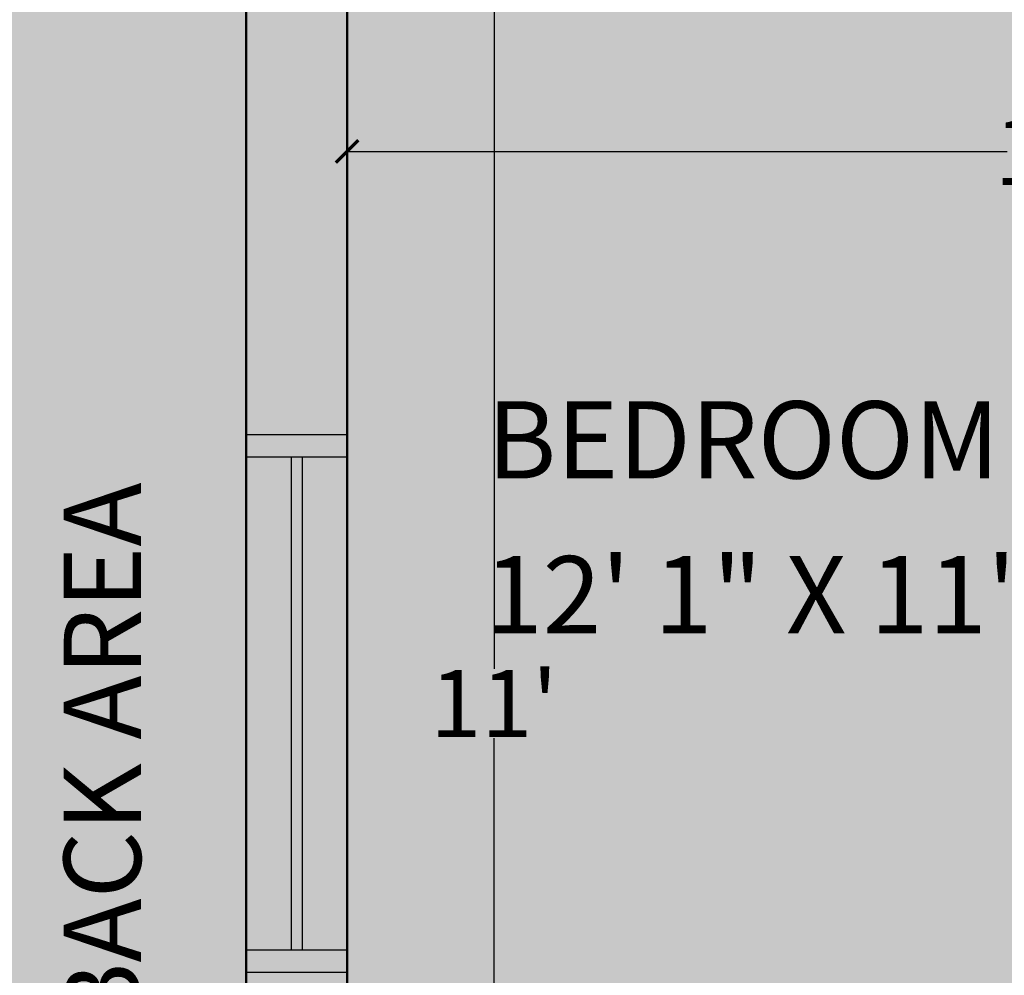
# Model space of a CAD drawing. Units: inches. Extents: x 528 to 2620, y -1066 to 798.
# Tile 7 of 41: x 600 to 688, y 620 to 705. Entities that reach past the tile are written whole.
import ezdxf

# ---------------------------------------------------------------- set-up
doc = ezdxf.new("R2010")
doc.units = ezdxf.units.IN
doc.header["$MEASUREMENT"] = 0
for name, color, linetype, lineweight in [('A-ANNO-DIMS', 2, 'Continuous', 18), ('A-AREA-IDEN', 7, 'Continuous', 18), ('A-GLAZ', 3, 'Continuous', 25), ('A-WALL', 7, 'Continuous', 50), ('A-WALL-PATT', 8, 'Continuous', 13)]:
    doc.layers.add(name, color=color, linetype=linetype, lineweight=lineweight)
doc.styles.get("Standard").update_dxf_attribs({"font": 'arial.ttf'})
doc.dimstyles.get("Standard").update_dxf_attribs({"dimtxt": 6, "dimasz": 2, "dimexe": 0.18, "dimexo": 0.0625, "dimgap": 0.09, "dimtad": 0, "dimtih": 1, "dimtoh": 1, "dimdec": 1, "dimzin": 0, "dimdsep": 46, "dimlunit": 3, "dimtxsty": 'Standard', "dimblk": 'ARCHTICK', "dimcen": 0.09, "dimadec": 0, "dimazin": 0, "dimtfac": 1, "dimtdec": 1, "dimtofl": 0, "dimtmove": 0, "dimatfit": 3, "dimfxl": 1, "dimtolj": 1, "dimtzin": 0, "dimarcsym": 0})

# ---------------------------------------------------------------- blocks, each defined once
blk = doc.blocks.new('_ArchTick')
at = {"color": 0, "linetype": 'ByBlock', "const_width": 0.15}
blk.add_lwpolyline([(-0.5, -0.5), (0.5, 0.5)], dxfattribs=at)
blk = doc.blocks.new('*D25')
at = {"layer": 'A-ANNO-DIMS', "color": 0, "lineweight": -2, "transparency": 16777216}
for p, q in [((629.059, 693.763), (629.059, 693.001)), ((774.059, 693.763), (774.059, 693.001)), ((629.059, 693.181), (687.951, 693.181)), ((774.059, 693.181), (715.168, 693.181))]:
    blk.add_line(p, q, dxfattribs=at)
at = {"layer": 'Defpoints', "color": 0, "transparency": 16777216}
for p in [(629.059, 693.826), (774.059, 693.826), (774.059, 693.181)]:
    blk.add_point(p, dxfattribs=at)
at = {"layer": 'A-ANNO-DIMS', "color": 0, "lineweight": -2, "transparency": 16777216, "xscale": 2, "yscale": 2, "zscale": 2, "rotation": 180}
blk.add_blockref('_ArchTick', (629.059, 693.181), dxfattribs=at)
at = {"layer": 'A-ANNO-DIMS', "color": 0, "lineweight": -2, "transparency": 16777216, "xscale": 2, "yscale": 2, "zscale": 2}
blk.add_blockref('_ArchTick', (774.059, 693.181), dxfattribs=at)
at = {"layer": 'A-ANNO-DIMS', "color": 0, "transparency": 16777216, "insert": (701.559, 693.181), "char_height": 6, "attachment_point": 5}
blk.add_mtext('\\A1;12\'-1.0"', dxfattribs=at)
blk = doc.blocks.new('*D26')
at = {"layer": 'A-ANNO-DIMS', "color": 0, "lineweight": -2, "transparency": 16777216}
for p, q in [((642.51, 709.922), (641.988, 709.922)), ((642.168, 709.922), (642.168, 647.025)), ((642.168, 577.922), (642.168, 640.82)), ((642.51, 577.922), (641.988, 577.922))]:
    blk.add_line(p, q, dxfattribs=at)
at = {"layer": 'Defpoints', "color": 0, "transparency": 16777216}
for p in [(642.572, 709.922), (642.168, 577.922), (642.572, 577.922)]:
    blk.add_point(p, dxfattribs=at)
at = {"layer": 'A-ANNO-DIMS', "color": 0, "lineweight": -2, "transparency": 16777216, "xscale": 2, "yscale": 2, "zscale": 2}
for p, rotation in [((642.168, 709.922), 90), ((642.168, 577.922), 270)]:
    blk.add_blockref('_ArchTick', p, dxfattribs=dict(at, rotation=rotation))
at = {"layer": 'A-ANNO-DIMS', "color": 0, "transparency": 16777216, "insert": (642.168, 643.922), "char_height": 6, "attachment_point": 5}
blk.add_mtext("\\A1;11'", dxfattribs=at)
blk = doc.blocks.new('WIN-1200')
for p, q in [((677.559, 718.922), (725.559, 718.922)), ((677.559, 709.922), (677.559, 718.922)), ((679.559, 709.922), (679.559, 718.922)), ((723.559, 718.922), (723.559, 709.922)), ((725.559, 718.922), (725.559, 709.922)), ((679.559, 714.922), (723.559, 714.922)), ((679.559, 713.922), (723.559, 713.922)), ((725.559, 709.922), (677.559, 709.922))]:
    blk.add_line(p, q)

msp = doc.modelspace()

# ---------------------------------------------------------------- hatches: boundary and pattern name
at = {"layer": 'A-WALL-PATT', "transparency": 33554475}
h = msp.add_hatch(color=256, dxfattribs=at)
h.dxf.hatch_style = 1
h.paths.add_polyline_path([(620.059, 718.922), (908.059, 718.922), (908.059, 268.922), (770.059, 268.922), (770.059, 220.922), (932.059, 220.922), (932.059, 741.922), (596.059, 741.922), (596.059, 391.422), (620.059, 391.422)])
at = {"layer": 'A-WALL-PATT', "transparency": 33554687}
h = msp.add_hatch(color=256, dxfattribs=at)
h.dxf.hatch_style = 1
h.paths.add_polyline_path([(861.059, 273.922), (817.059, 273.922), (817.059, 272.922), (861.059, 272.922)])
h.paths.add_polyline_path([(817.059, 277.922), (815.059, 277.922), (815.059, 268.922), (817.059, 268.922)])
h.paths.add_polyline_path([(908.059, 397.922), (899.059, 397.922), (899.059, 395.922), (908.059, 395.922)])
h.paths.add_polyline_path([(908.059, 443.922), (899.059, 443.922), (899.059, 441.922), (908.059, 441.922)])
h.paths.add_polyline_path([(904.059, 441.922), (903.059, 441.922), (903.059, 397.922), (904.059, 397.922)])
h.paths.add_polyline_path([(625.059, 561.422), (624.059, 561.422), (624.059, 537.422), (625.059, 537.422)])
h.paths.add_polyline_path([(648.747, 334.444), (720.045, 334.444), (720.045, 344.998), (648.747, 344.998)], flags=9)
h.paths.add_polyline_path([(819.733, 323.153), (880.328, 323.153), (880.328, 333.708), (819.733, 333.708)], flags=9)
h.paths.add_polyline_path([(779.898, 680.607), (821.764, 680.607), (821.764, 691.169), (779.898, 691.169)], flags=9)
h.paths.add_polyline_path([(779.876, 692.362), (817.138, 692.362), (817.138, 703.058), (779.876, 703.058)], flags=9)
h.paths.add_polyline_path([(799.994, 453.884), (860.589, 453.884), (860.589, 464.439), (799.994, 464.439)], flags=9)
h.paths.add_polyline_path([(650.866, 539.397), (708.781, 539.397), (708.781, 549.952), (650.866, 549.952)], flags=9)
h.paths.add_polyline_path([(788.504, 612.01), (849.099, 612.01), (849.099, 622.565), (788.504, 622.565)], flags=9)
h.paths.add_polyline_path([(639.539, 648.31), (700.134, 648.31), (700.134, 658.865), (639.539, 658.865)], flags=9)
h.paths.add_polyline_path([(648.913, 346.09), (747.706, 346.09), (747.706, 356.778), (648.913, 356.778)], flags=9)
h.paths.add_polyline_path([(676.857, 450.66), (746.735, 450.66), (746.735, 461.355), (676.857, 461.355)], flags=9)
h.paths.add_polyline_path([(819.711, 334.947), (865.526, 334.947), (865.526, 345.636), (819.711, 345.636)], flags=9)
h.paths.add_polyline_path([(806.298, 467.745), (874.047, 467.745), (874.047, 478.441), (806.298, 478.441)], flags=9)
h.paths.add_polyline_path([(653.235, 552.284), (690.497, 552.284), (690.497, 562.979), (653.235, 562.979)], flags=9)
h.paths.add_polyline_path([(789.903, 623.407), (843.208, 623.407), (843.208, 634.103), (789.903, 634.103)], flags=9)
h.paths.add_polyline_path([(639.773, 662.103), (693.077, 662.103), (693.077, 672.798), (639.773, 672.798)], flags=9)
h.paths.add_polyline_path([(801.587, 242.914), (846.334, 242.914), (846.334, 253.603), (801.587, 253.603)], flags=9)
h.paths.add_polyline_path([(925.362, 593.982), (925.362, 674.057), (914.673, 674.057), (914.673, 593.982)], flags=9)
h.paths.add_polyline_path([(612.559, 593.982), (612.559, 674.057), (601.871, 674.057), (601.871, 593.982)], flags=9)
h.paths.add_polyline_path([(723.31, 726.564), (803.385, 726.564), (803.385, 737.252), (723.31, 737.252)], flags=9)
at = {"layer": 'A-WALL-PATT', "transparency": 33554521}
h = msp.add_hatch(color=256, dxfattribs=at)
h.dxf.hatch_style = 1
h.paths.add_polyline_path([(629.059, 709.922), (677.559, 709.922), (677.559, 718.922), (620.059, 718.922), (620.059, 667.922), (629.059, 667.922)])
h.paths.add_polyline_path([(790.559, 718.922), (725.559, 718.922), (725.559, 709.922), (774.059, 709.922), (774.059, 577.922), (768.481, 577.922), (768.559, 573.422), (774.059, 573.422), (774.059, 567.422), (778.559, 567.422), (778.559, 669.422), (831.059, 669.422), (831.059, 675.922), (826.559, 675.922), (826.559, 673.922), (778.559, 673.922), (778.559, 709.922), (790.559, 709.922)])
h.paths.add_polyline_path([(908.059, 718.922), (879.059, 718.922), (879.059, 709.922), (899.059, 709.922), (899.059, 641.672), (908.059, 641.672)])
h.paths.add_polyline_path([(629.059, 619.922), (620.059, 619.922), (620.059, 561.422), (629.059, 561.422), (629.059, 573.422), (724.059, 573.422), (724.059, 569.422), (728.559, 569.422), (728.559, 577.922), (629.059, 577.922)])
h.paths.add_polyline_path([(779.059, 391.422), (779.059, 400.422), (770.059, 400.422), (764.059, 400.422), (764.059, 397.422), (764.059, 391.422), (770.059, 391.422), (770.059, 268.922), (815.059, 268.922), (815.059, 277.922), (779.059, 277.922), (779.059, 359.767)])
h.paths.add_polyline_path([(908.059, 395.922), (899.059, 395.922), (851.059, 395.922), (851.059, 391.422), (899.059, 391.422), (899.059, 277.922), (863.059, 277.922), (863.059, 268.922), (908.059, 268.922)])
h.paths.add_polyline_path([(908.059, 593.672), (899.059, 593.672), (899.059, 525.422), (778.559, 525.422), (778.559, 527.172), (774.059, 527.172), (774.059, 520.922), (899.059, 520.922), (899.059, 443.922), (908.059, 443.922)])
h.paths.add_polyline_path([(629.059, 520.922), (728.559, 520.922), (728.559, 545.422), (724.059, 545.422), (724.059, 525.422), (629.059, 525.422), (629.059, 537.422), (620.059, 537.422), (620.059, 484.672), (629.059, 484.672)])
h.paths.add_polyline_path([(629.059, 436.672), (620.059, 436.672), (620.059, 391.422), (648.559, 391.422), (648.559, 400.422), (629.059, 400.422)])
h.paths.add_polyline_path([(716.059, 397.422), (716.059, 400.422), (696.559, 400.422), (696.559, 391.422), (716.059, 391.422)])
at = {"layer": 'A-WALL-PATT', "transparency": 33554681}
h = msp.add_hatch(color=256, dxfattribs=at)
h.dxf.hatch_style = 1
h.paths.add_polyline_path([(629.059, 665.922), (625.059, 665.922), (625.059, 621.922), (629.059, 621.922)])
h.paths.add_polyline_path([(624.059, 665.922), (620.059, 665.922), (620.059, 621.922), (624.059, 621.922)])
h.paths.add_polyline_path([(723.559, 713.922), (679.559, 713.922), (679.559, 709.922), (723.559, 709.922)])
h.paths.add_polyline_path([(723.559, 718.922), (679.559, 718.922), (679.559, 714.922), (723.559, 714.922)])
h.paths.add_polyline_path([(814.559, 713.922), (790.559, 713.922), (790.559, 709.922), (814.559, 709.922)])
h.paths.add_polyline_path([(814.559, 718.922), (790.559, 718.922), (790.559, 714.922), (814.559, 714.922)])
h.paths.add_polyline_path([(877.059, 713.922), (833.059, 713.922), (833.059, 709.922), (877.059, 709.922)])
h.paths.add_polyline_path([(877.059, 718.922), (833.059, 718.922), (833.059, 714.922), (877.059, 714.922)])
h.paths.add_polyline_path([(908.059, 639.672), (904.059, 639.672), (904.059, 595.672), (908.059, 595.672)])
h.paths.add_polyline_path([(903.059, 639.672), (899.059, 639.672), (899.059, 595.672), (903.059, 595.672)])
h.paths.add_polyline_path([(908.059, 441.922), (904.059, 441.922), (904.059, 397.922), (908.059, 397.922)])
h.paths.add_polyline_path([(903.059, 441.922), (899.059, 441.922), (899.059, 397.922), (903.059, 397.922)])
h.paths.add_polyline_path([(861.059, 272.922), (817.059, 272.922), (817.059, 268.922), (861.059, 268.922)])
h.paths.add_polyline_path([(861.059, 277.922), (817.059, 277.922), (817.059, 273.922), (861.059, 273.922)])
h.paths.add_polyline_path([(694.559, 395.422), (650.559, 395.422), (650.559, 391.422), (694.559, 391.422)])
h.paths.add_polyline_path([(694.559, 400.422), (650.559, 400.422), (650.559, 396.422), (694.559, 396.422)])
h.paths.add_polyline_path([(629.059, 482.672), (625.059, 482.672), (625.059, 438.672), (629.059, 438.672)])
h.paths.add_polyline_path([(624.059, 482.672), (620.059, 482.672), (620.059, 438.672), (624.059, 438.672)])
h.paths.add_polyline_path([(629.059, 561.422), (625.059, 561.422), (625.059, 537.422), (629.059, 537.422)])
h.paths.add_polyline_path([(624.059, 561.422), (620.059, 561.422), (620.059, 537.422), (624.059, 537.422)])
h = msp.add_hatch(color=256, dxfattribs=at)
h.dxf.hatch_style = 1
h.paths.add_polyline_path([(625.059, 665.922), (624.059, 665.922), (624.059, 621.922), (625.059, 621.922)])
h.paths.add_polyline_path([(629.059, 667.922), (620.059, 667.922), (620.059, 665.922), (629.059, 665.922)])
h.paths.add_polyline_path([(629.059, 621.922), (620.059, 621.922), (620.059, 619.922), (629.059, 619.922)])
h.paths.add_polyline_path([(723.559, 714.922), (679.559, 714.922), (679.559, 713.922), (723.559, 713.922)])
h.paths.add_polyline_path([(725.559, 718.922), (723.559, 718.922), (723.559, 709.922), (725.559, 709.922)])
h.paths.add_polyline_path([(679.559, 718.922), (677.559, 718.922), (677.559, 709.922), (679.559, 709.922)])
h.paths.add_polyline_path([(814.559, 714.922), (790.559, 714.922), (790.559, 713.922), (814.559, 713.922)])
h.paths.add_polyline_path([(877.059, 714.922), (833.059, 714.922), (833.059, 713.922), (877.059, 713.922)])
h.paths.add_polyline_path([(879.059, 718.922), (877.059, 718.922), (877.059, 709.922), (879.059, 709.922)])
h.paths.add_polyline_path([(833.059, 718.922), (831.059, 718.922), (831.059, 709.922), (833.059, 709.922)])
h.paths.add_polyline_path([(650.559, 400.422), (648.559, 400.422), (648.559, 391.422), (650.559, 391.422)])
h.paths.add_polyline_path([(694.559, 396.422), (650.559, 396.422), (650.559, 395.422), (694.559, 395.422)])
h.paths.add_polyline_path([(696.559, 400.422), (694.559, 400.422), (694.559, 391.422), (696.559, 391.422)])
h.paths.add_polyline_path([(629.059, 438.672), (620.059, 438.672), (620.059, 436.672), (629.059, 436.672)])
h.paths.add_polyline_path([(629.059, 484.672), (620.059, 484.672), (620.059, 482.672), (629.059, 482.672)])
h.paths.add_polyline_path([(625.059, 482.672), (624.059, 482.672), (624.059, 438.672), (625.059, 438.672)])
at = {"layer": 'A-WALL-PATT', "transparency": 33554590}
h = msp.add_hatch(color=256, dxfattribs=at)
h.dxf.hatch_style = 1
h.paths.add_polyline_path([(774.059, 709.922), (629.059, 709.922), (629.059, 577.922), (728.559, 577.922), (728.559, 579.422), (728.559, 619.422), (730.309, 619.422), (730.309, 619.384, -0.401453), (768.559, 579.422), (768.559, 577.922), (774.059, 577.922)])
h.paths.add_polyline_path([(723.896, 686.058), (723.968, 686.064), (723.828, 686.128)], flags=0)
h.paths.add_polyline_path([(722.785, 642.699), (722.893, 642.756), (722.893, 684.992), (722.647, 685.244), (722.647, 685.82), (723.079, 686.262), (723.533, 686.262), (723.968, 686.064), (724.739, 686.128), (770.696, 686.128), (770.78, 686.14), (771.126, 686.266), (771.694, 686.094), (771.94, 685.478), (771.67, 684.904), (771.582, 684.871), (771.582, 642.782), (771.878, 642.514), (771.878, 641.921), (771.511, 641.462), (770.855, 641.462), (770.401, 641.833), (770.401, 641.551), (724.739, 641.551), (723.991, 641.705), (723.443, 641.414), (722.879, 641.585), (722.597, 642.142)], flags=16)
h.paths.add_polyline_path([(723.994, 641.704), (723.994, 641.707), (723.991, 641.705)], flags=0)
h.paths.add_polyline_path([(722.893, 642.732), (722.893, 684.992), (722.647, 685.244), (722.647, 685.82), (723.079, 686.262), (723.287, 686.262), (722.991, 686.172), (722.794, 685.971), (722.647, 685.68), (722.647, 685.434), (722.745, 685.143), (722.942, 684.942), (723.238, 684.807), (723.484, 684.807), (723.779, 684.897), (723.976, 685.098), (724.174, 685.488), (724.124, 685.635), (724.124, 685.249), (723.631, 684.746), (723.631, 642.961), (724.124, 642.514), (724.124, 641.887), (723.656, 641.462), (723.079, 641.462), (722.647, 641.904), (722.647, 642.48)], flags=0)
h.paths.add_polyline_path([(722.647, 642.29), (722.647, 642.044), (722.794, 641.753), (723.079, 641.462), (723.287, 641.462), (722.879, 641.585), (722.597, 642.142)], flags=0)
h.paths.add_polyline_path([(770.745, 686.128), (770.58, 686.128), (770.551, 686.057)], flags=0)
h.paths.add_polyline_path([(743.299, 645.288), (753.227, 659.398), (748.69, 663.75), (753.234, 668.538), (743.299, 682.458), (743.791, 682.592), (744.136, 682.681), (744.53, 682.928), (744.628, 683.084), (745.017, 683.327), (744.53, 684.069), (744.776, 684.158), (744.874, 684.315), (745.514, 684.404), (746.081, 684.651), (746.474, 684.651), (746.819, 684.807), (747.459, 685.031), (747.705, 685.143), (748.198, 685.277), (748.394, 685.523), (748.862, 685.523), (749.994, 686.128), (753.488, 676.03), (757.379, 680.153), (757.791, 679.758), (758.044, 680.645), (758.29, 681.227), (758.29, 682.055), (758.019, 682.592), (757.871, 683.174), (757.822, 683.778), (758.388, 684.069), (758.979, 684.203), (759.619, 684.158), (760.21, 683.957), (760.751, 683.666), (761.859, 683.666), (762.401, 683.957), (762.991, 684.114), (763.631, 684.114), (764.198, 683.957), (764.739, 683.666), (766.118, 683.666), (766.659, 683.957), (767.25, 684.158), (767.865, 684.203), (768.456, 684.069), (769.047, 683.778), (768.998, 683.174), (768.85, 682.592), (768.554, 682.055), (768.554, 681.227), (768.801, 680.645), (769.092, 679.75), (768.948, 678.832), (768.801, 678.228), (768.554, 677.646), (768.554, 676.818), (768.801, 676.237), (769.092, 675.341), (768.948, 674.424), (768.801, 673.82), (768.554, 673.283), (768.554, 672.41), (768.801, 671.873), (768.998, 671.291), (769.047, 670.642), (768.948, 670.016), (768.801, 669.411), (768.554, 668.874), (768.554, 668.002), (768.974, 667.239), (769.047, 666.279), (769.047, 665.563), (768.456, 665.316), (767.865, 665.16), (767.25, 665.16), (766.659, 665.361), (766.118, 665.697), (764.739, 665.697), (763.945, 665.204), (762.991, 665.204), (762.401, 665.361), (761.859, 665.697), (761.005, 665.697), (762.696, 664.086), (760.741, 662.027), (761.859, 662.027), (762.401, 662.318), (763.342, 662.548), (764.247, 662.318), (764.788, 662.027), (766.118, 662.027), (766.659, 662.318), (767.25, 662.519), (767.865, 662.564), (768.505, 662.43), (769.047, 662.116), (769.047, 661.4), (769.047, 660.796), (768.85, 660.214), (768.554, 659.677), (768.554, 658.849), (768.85, 658.267), (768.998, 657.663), (769.069, 656.749), (768.85, 655.851), (768.554, 655.269), (768.554, 654.441), (768.85, 653.859), (769.069, 652.961), (768.998, 652.046), (768.85, 651.442), (768.554, 650.905), (768.554, 650.032), (768.85, 649.495), (768.998, 648.914), (769.047, 648.265), (768.998, 647.638), (768.85, 647.034), (768.554, 646.497), (768.554, 645.624), (768.85, 645.087), (769.047, 644.55), (769.047, 643.901), (768.505, 643.655), (767.865, 643.521), (767.25, 643.521), (766.659, 643.722), (766.118, 644.058), (764.788, 644.058), (764.247, 643.722), (763.342, 643.492), (762.401, 643.722), (761.859, 644.058), (760.801, 644.058), (760.259, 643.722), (759.668, 643.521), (759.028, 643.521), (758.388, 643.655), (757.871, 643.901), (757.871, 644.55), (758.044, 645.087), (758.339, 645.624), (758.339, 646.497), (758.044, 647.034), (757.921, 647.638), (757.866, 648.059), (757.379, 647.593), (753.422, 651.773), (749.994, 641.618), (749.502, 641.708), (749.354, 641.954), (748.542, 642.446), (747.311, 642.939), (746.652, 642.939), (746.327, 643.185), (745.514, 643.565), (744.53, 643.655), (745.011, 644.4), (744.628, 644.639), (744.136, 644.886), (743.791, 645.132)], flags=0)
h.paths.add_polyline_path([(755.656, 654.933), (756.542, 654.687), (757.527, 654.329), (756.641, 654.575)], flags=0)
h.paths.add_polyline_path([(758.339, 649.204), (758.339, 648.712), (758.585, 644.304), (758.585, 648.802)], flags=0)
h.paths.add_polyline_path([(758.339, 649.294), (758.093, 649.697), (758.359, 649.165)], flags=0)
h.paths.add_polyline_path([(755.656, 672.79), (756.493, 673.037), (757.358, 673.351), (757.353, 673.358), (756.641, 673.149)], flags=0)
h.paths.add_polyline_path([(760.264, 639.641), (771.408, 639.641), (771.408, 624.039), (760.264, 624.039)], flags=16)
h.paths.add_polyline_path([(761.378, 638.526), (770.294, 638.526), (770.294, 625.153), (761.378, 625.153)], flags=0)
edge = h.paths.add_edge_path(flags=0)
edge.add_ellipse((765.836, 631.84), major_axis=(-2.245, 2.245), ratio=1, start_angle=-45, end_angle=45, ccw=False)
edge.add_ellipse((765.836, 631.84), major_axis=(-2.245, 2.245), ratio=1, start_angle=-135, end_angle=-45, ccw=False)
edge.add_ellipse((765.836, 631.84), major_axis=(-2.245, 2.245), ratio=1, start_angle=135, end_angle=-135, ccw=False)
edge.add_ellipse((765.836, 631.84), major_axis=(-2.245, 2.245), ratio=1, start_angle=45, end_angle=135, ccw=False)
h.paths.add_polyline_path([(758.585, 683.42), (758.585, 678.922), (758.373, 678.575), (758.339, 678.43), (758.093, 678.049), (758.339, 678.519), (758.339, 679.011)], flags=0)
h.paths.add_polyline_path([(760.264, 688.038), (760.264, 703.64), (771.408, 703.64), (771.408, 688.038)], flags=16)
h.paths.add_polyline_path([(770.401, 685.389), (770.401, 685.846), (770.855, 686.217), (771.511, 686.217), (771.878, 685.758), (771.878, 685.165), (771.582, 684.897), (771.582, 642.782), (771.878, 642.514), (771.878, 641.921), (771.511, 641.462), (770.855, 641.462), (770.401, 641.833), (770.401, 642.29)], flags=0)
h.paths.add_polyline_path([(770.532, 642.678), (771.052, 643.009), (771.67, 642.775), (771.94, 642.201), (771.694, 641.585), (771.126, 641.413), (770.551, 641.622), (770.347, 642.132)], flags=16)
h.paths.add_polyline_path([(761.378, 689.152), (761.378, 702.526), (770.294, 702.526), (770.294, 689.152)], flags=0)
edge = h.paths.add_edge_path(flags=0)
edge.add_ellipse((765.836, 695.839), major_axis=(2.245, 2.245), ratio=1, start_angle=405, end_angle=495, ccw=False)
edge.add_ellipse((765.836, 695.839), major_axis=(2.245, 2.245), ratio=1, start_angle=675, end_angle=765, ccw=False)
edge.add_ellipse((765.836, 695.839), major_axis=(2.245, 2.245), ratio=1, start_angle=585, end_angle=675, ccw=False)
edge.add_ellipse((765.836, 695.839), major_axis=(2.245, 2.245), ratio=1, start_angle=495, end_angle=585, ccw=False)
h.paths.add_polyline_path([(770.696, 684.897), (770.942, 684.74), (771.41, 684.74), (771.73, 685.031), (771.878, 685.344), (771.878, 685.635), (771.694, 686.094), (771.582, 686.128), (771.878, 685.758), (771.878, 685.165), (771.41, 684.74), (770.849, 684.74)], flags=0)
h.paths.add_polyline_path([(899.059, 709.922), (831.059, 709.922), (831.059, 699.922), (829.809, 699.922), (829.809, 675.922), (831.059, 675.922), (831.059, 669.422), (778.559, 669.422), (778.559, 567.172), (780.059, 567.172), (820.059, 567.172), (820.059, 565.422), (820.021, 565.422, -0.401453), (780.059, 527.172), (778.559, 527.172), (778.559, 525.422), (899.059, 525.422)])
h.paths.add_polyline_path([(849.197, 636.014), (849.269, 636.02), (849.129, 636.084)], flags=0)
h.paths.add_polyline_path([(848.193, 634.948), (847.947, 635.2), (847.947, 635.776), (848.379, 636.218), (848.833, 636.218), (849.269, 636.02), (850.039, 636.084), (895.996, 636.084), (896.081, 636.096), (896.426, 636.222), (896.995, 636.05), (897.241, 635.434), (896.97, 634.86), (896.883, 634.827), (896.883, 592.738), (897.178, 592.47), (897.178, 591.877), (896.811, 591.418), (896.155, 591.418), (895.701, 591.789), (895.701, 591.507), (850.039, 591.507), (849.292, 591.661), (848.744, 591.37), (848.18, 591.541), (847.897, 592.098), (848.086, 592.655), (848.193, 592.712)], flags=16)
h.paths.add_polyline_path([(849.294, 591.66), (849.295, 591.663), (849.292, 591.661)], flags=16)
h.paths.add_polyline_path([(848.193, 634.948), (847.947, 635.2), (847.947, 635.776), (848.379, 636.218), (848.587, 636.218), (848.292, 636.128), (848.095, 635.927), (847.947, 635.636), (847.947, 635.39), (848.046, 635.099), (848.243, 634.897), (848.538, 634.763), (848.784, 634.763), (849.079, 634.853), (849.276, 635.054), (849.474, 635.444), (849.424, 635.591), (849.424, 635.205), (848.932, 634.702), (848.932, 592.917), (849.424, 592.47), (849.424, 591.843), (848.956, 591.418), (848.379, 591.418), (847.947, 591.86), (847.947, 592.436), (848.193, 592.688)], flags=0)
h.paths.add_polyline_path([(847.947, 592.246), (847.947, 592), (848.095, 591.709), (848.379, 591.418), (848.587, 591.418), (848.18, 591.541), (847.897, 592.098)], flags=16)
h.paths.add_polyline_path([(896.046, 636.084), (895.88, 636.084), (895.852, 636.013)], flags=0)
h.paths.add_polyline_path([(868.599, 632.414), (869.092, 632.548), (869.436, 632.637), (869.83, 632.884), (869.929, 633.04), (870.318, 633.283), (869.83, 634.025), (870.076, 634.114), (870.175, 634.271), (870.815, 634.36), (871.381, 634.607), (871.775, 634.607), (872.119, 634.763), (872.759, 634.987), (873.006, 635.099), (873.498, 635.233), (873.695, 635.479), (874.163, 635.479), (875.295, 636.084), (878.788, 625.986), (882.679, 630.109), (883.091, 629.714), (883.344, 630.601), (883.59, 631.183), (883.59, 632.011), (883.319, 632.548), (883.172, 633.13), (883.123, 633.734), (883.689, 634.025), (884.279, 634.159), (884.919, 634.114), (885.51, 633.913), (886.052, 633.622), (887.159, 633.622), (887.701, 633.913), (888.292, 634.07), (888.932, 634.07), (889.498, 633.913), (890.039, 633.622), (891.418, 633.622), (891.959, 633.913), (892.55, 634.114), (893.166, 634.159), (893.756, 634.025), (894.347, 633.734), (894.298, 633.13), (894.15, 632.548), (893.855, 632.011), (893.855, 631.183), (894.101, 630.601), (894.393, 629.706), (894.249, 628.788), (894.101, 628.184), (893.855, 627.602), (893.855, 626.774), (894.101, 626.193), (894.393, 625.297), (894.249, 624.38), (894.101, 623.776), (893.855, 623.239), (893.855, 622.366), (894.101, 621.829), (894.298, 621.247), (894.347, 620.598), (894.249, 619.972), (894.101, 619.367), (893.855, 618.83), (893.855, 617.958), (894.274, 617.195), (894.347, 616.235), (894.347, 615.518), (893.756, 615.272), (893.166, 615.116), (892.55, 615.116), (891.959, 615.317), (891.418, 615.653), (890.039, 615.653), (889.245, 615.16), (888.292, 615.16), (887.701, 615.317), (887.159, 615.653), (886.305, 615.653), (887.996, 614.042), (886.041, 611.983), (887.159, 611.983), (887.701, 612.274), (888.642, 612.504), (889.547, 612.274), (890.089, 611.983), (891.418, 611.983), (891.959, 612.274), (892.55, 612.475), (893.166, 612.52), (893.806, 612.386), (894.347, 612.072), (894.347, 611.356), (894.347, 610.752), (894.15, 610.17), (893.855, 609.633), (893.855, 608.805), (894.15, 608.223), (894.298, 607.619), (894.37, 606.705), (894.15, 605.807), (893.855, 605.225), (893.855, 604.397), (894.15, 603.815), (894.37, 602.917), (894.298, 602.002), (894.15, 601.398), (893.855, 600.861), (893.855, 599.988), (894.15, 599.451), (894.298, 598.87), (894.347, 598.221), (894.298, 597.594), (894.15, 596.99), (893.855, 596.453), (893.855, 595.58), (894.15, 595.043), (894.347, 594.506), (894.347, 593.857), (893.806, 593.611), (893.166, 593.477), (892.55, 593.477), (891.959, 593.678), (891.418, 594.014), (890.089, 594.014), (889.547, 593.678), (888.642, 593.448), (887.701, 593.678), (887.159, 594.014), (886.101, 594.014), (885.559, 593.678), (884.969, 593.477), (884.329, 593.477), (883.689, 593.611), (883.172, 593.857), (883.172, 594.506), (883.344, 595.043), (883.639, 595.58), (883.639, 596.453), (883.344, 596.99), (883.221, 597.594), (883.167, 598.015), (882.679, 597.549), (878.722, 601.729), (875.295, 591.574), (874.803, 591.664), (874.655, 591.91), (873.843, 592.402), (872.612, 592.895), (871.952, 592.895), (871.627, 593.141), (870.815, 593.521), (869.83, 593.611), (870.311, 594.356), (869.929, 594.595), (869.436, 594.842), (869.092, 595.088), (868.599, 595.244), (878.528, 609.354), (873.99, 613.706), (878.535, 618.494)], flags=0)
h.paths.add_polyline_path([(880.956, 622.746), (881.793, 622.993), (882.659, 623.307), (882.654, 623.314), (881.941, 623.104)], flags=0)
h.paths.add_polyline_path([(880.956, 604.889), (881.843, 604.643), (882.827, 604.285), (881.941, 604.531)], flags=16)
h.paths.add_polyline_path([(883.393, 628.005), (883.639, 628.475), (883.639, 628.967), (883.886, 633.376), (883.886, 628.878), (883.674, 628.531), (883.639, 628.386)], flags=0)
h.paths.add_polyline_path([(883.639, 599.16), (883.639, 598.668), (883.886, 594.26), (883.886, 598.758)], flags=16)
h.paths.add_polyline_path([(883.639, 599.25), (883.393, 599.653), (883.659, 599.121)], flags=16)
h.paths.add_polyline_path([(885.564, 637.994), (885.564, 653.596), (896.709, 653.596), (896.709, 637.994)], flags=16)
h.paths.add_polyline_path([(885.564, 589.597), (896.709, 589.597), (896.709, 573.995), (885.564, 573.995)], flags=16)
h.paths.add_polyline_path([(886.679, 639.108), (886.679, 652.482), (895.594, 652.482), (895.594, 639.108)], flags=0)
h.paths.add_polyline_path([(886.679, 588.482), (895.594, 588.482), (895.594, 575.109), (886.679, 575.109)], flags=0)
edge = h.paths.add_edge_path(flags=0)
edge.add_ellipse((891.136, 645.795), major_axis=(2.245, 2.245), ratio=1, start_angle=405, end_angle=495, ccw=False)
edge.add_ellipse((891.136, 645.795), major_axis=(2.245, 2.245), ratio=1, start_angle=675, end_angle=765, ccw=False)
edge.add_ellipse((891.136, 645.795), major_axis=(2.245, 2.245), ratio=1, start_angle=585, end_angle=675, ccw=False)
edge.add_ellipse((891.136, 645.795), major_axis=(2.245, 2.245), ratio=1, start_angle=495, end_angle=585, ccw=False)
edge = h.paths.add_edge_path(flags=0)
edge.add_ellipse((891.136, 581.796), major_axis=(-2.245, 2.245), ratio=1, start_angle=-45, end_angle=45, ccw=False)
edge.add_ellipse((891.136, 581.796), major_axis=(-2.245, 2.245), ratio=1, start_angle=-135, end_angle=-45, ccw=False)
edge.add_ellipse((891.136, 581.796), major_axis=(-2.245, 2.245), ratio=1, start_angle=135, end_angle=-135, ccw=False)
edge.add_ellipse((891.136, 581.796), major_axis=(-2.245, 2.245), ratio=1, start_angle=45, end_angle=135, ccw=False)
h.paths.add_polyline_path([(895.701, 635.345), (895.701, 635.802), (896.155, 636.173), (896.811, 636.173), (897.178, 635.714), (897.178, 635.121), (896.883, 634.853), (896.883, 592.738), (897.178, 592.47), (897.178, 591.877), (896.811, 591.418), (896.155, 591.418), (895.701, 591.789), (895.701, 592.246)], flags=0)
h.paths.add_polyline_path([(895.996, 634.853), (896.243, 634.696), (896.71, 634.696), (897.03, 634.987), (897.178, 635.3), (897.178, 635.591), (896.995, 636.05), (896.883, 636.084), (897.178, 635.714), (897.178, 635.121), (896.71, 634.696), (896.15, 634.696)], flags=0)
h.paths.add_polyline_path([(895.832, 592.634), (896.353, 592.965), (896.97, 592.731), (897.241, 592.157), (896.995, 591.541), (896.426, 591.369), (895.852, 591.578), (895.648, 592.088)], flags=16)
h.paths.add_polyline_path([(725.255, 569.422), (724.059, 569.422), (724.059, 573.422), (629.059, 573.422), (629.059, 525.422), (724.059, 525.422), (724.059, 545.422), (725.255, 545.422)])
h.paths.add_polyline_path([(820.021, 565.422), (780.059, 565.422), (780.059, 567.172), (774.059, 567.172), (774.059, 567.422), (774.059, 573.422), (768.559, 573.422), (768.481, 577.922), (768.559, 577.922), (768.559, 579.422, 0.401453), (730.309, 619.384), (730.309, 579.422), (728.559, 579.422), (728.559, 573.422), (728.559, 569.422), (727.255, 569.422), (727.255, 545.422), (728.559, 545.422), (728.559, 520.922), (665.059, 520.922), (665.059, 436.422), (716.059, 436.422), (716.059, 421.422), (717.809, 421.422), (717.809, 421.358, -0.392996), (740.059, 397.422, -0.392996), (762.309, 421.358), (762.309, 421.422), (764.059, 421.422), (764.059, 400.422), (770.059, 400.422), (779.059, 400.422), (779.059, 391.422), (779.059, 359.767), (795.432, 359.767), (795.432, 294.295), (893.669, 294.295), (893.669, 277.922), (899.059, 277.922), (899.059, 391.422), (851.059, 391.422), (851.059, 395.922), (899.059, 395.922), (899.059, 443.922), (899.059, 520.922), (774.059, 520.922), (774.059, 527.172), (778.559, 527.172), (780.059, 527.172, 0.401453)])
h.paths.add_polyline_path([(774.059, 519.657), (842.122, 519.657), (842.122, 505.072), (788.644, 505.072), (788.644, 474.079), (788.644, 470.433, -0.883215), (779.529, 456.663), (774.971, 456.663, -0.414214), (774.059, 457.575)], flags=16)
h.paths.add_polyline_path([(775.883, 517.834), (840.299, 517.834), (840.299, 514.188), (788.644, 514.188), (788.644, 484.41), (779.529, 484.41), (779.529, 474.079), (775.883, 474.079)], flags=0)
h.paths.add_polyline_path([(706.7, 501.564, -0.254069), (706.7, 493.021), (698.31, 492.555), (698.31, 502.031)], flags=16)
h.paths.add_polyline_path([(691.334, 515.692), (691.8, 507.301), (682.325, 507.301), (682.791, 515.692, -0.254069)], flags=16)
h.paths.add_polyline_path([(695.485, 504.685), (695.485, 479.416), (678.64, 479.416), (678.64, 504.685)], flags=16)
h.paths.add_polyline_path([(706.7, 489.602, -0.254069), (706.7, 481.058), (698.31, 480.592), (698.31, 490.068)], flags=16)
h.paths.add_polyline_path([(675.815, 502.031), (675.815, 492.555), (667.425, 493.021, -0.254069), (667.425, 501.564)], flags=16)
h.paths.add_polyline_path([(691.8, 476.8), (691.334, 468.409, -0.254069), (682.791, 468.409), (682.325, 476.8)], flags=16)
h.paths.add_polyline_path([(675.815, 490.068), (675.815, 480.592), (667.425, 481.058, -0.254069), (667.425, 489.602)], flags=16)
h.paths.add_polyline_path([(764.059, 397.422), (762.309, 397.422), (762.309, 421.358, 0.392996), (740.059, 397.422, 0.392996), (717.809, 421.358), (717.809, 397.422), (716.059, 397.422), (716.059, 391.422), (716.059, 385.422), (764.059, 385.422), (764.059, 391.422)], flags=17)
h.paths.add_polyline_path([(716.059, 436.422), (705.859, 436.422), (705.859, 418.422), (716.059, 418.422), (716.059, 421.422)], flags=17)
h.paths.add_polyline_path([(716.059, 418.422), (705.859, 418.422), (705.859, 400.422), (716.059, 400.422)], flags=17)
h.paths.add_polyline_path([(705.859, 418.422), (695.659, 418.422), (695.659, 400.422), (696.559, 400.422), (705.859, 400.422)], flags=17)
h.paths.add_polyline_path([(705.859, 436.422), (695.659, 436.422), (695.659, 418.422), (705.859, 418.422)], flags=17)
h.paths.add_polyline_path([(695.659, 418.422), (685.459, 418.422), (685.459, 400.422), (695.659, 400.422)], flags=17)
h.paths.add_polyline_path([(695.659, 436.422), (685.459, 436.422), (685.459, 418.422), (695.659, 418.422)], flags=17)
h.paths.add_polyline_path([(685.459, 418.422), (675.259, 418.422), (675.259, 400.422), (685.459, 400.422)], flags=17)
h.paths.add_polyline_path([(685.459, 436.422), (675.259, 436.422), (675.259, 418.422), (685.459, 418.422)], flags=17)
h.paths.add_polyline_path([(675.259, 436.422), (665.059, 436.422), (665.059, 418.422), (675.259, 418.422)])
h.paths.add_polyline_path([(675.259, 418.422), (665.059, 418.422), (665.059, 400.422), (675.259, 400.422)])
h.paths.add_polyline_path([(665.059, 418.422), (646.967, 418.422), (646.991, 436.422), (629.059, 436.422), (629.059, 400.422), (665.059, 400.422)])
h.paths.add_polyline_path([(665.059, 436.422), (646.991, 436.422), (646.967, 418.422), (665.059, 418.422)], flags=17)
h.paths.add_polyline_path([(647.005, 446.622), (629.059, 446.622), (629.059, 436.672), (629.059, 436.422), (646.991, 436.422)])
h.paths.add_polyline_path([(665.059, 446.622), (647.005, 446.622), (646.991, 436.422), (665.059, 436.422)])
h.paths.add_polyline_path([(647.019, 456.822), (629.059, 456.822), (629.059, 446.622), (647.005, 446.622)])
h.paths.add_polyline_path([(665.059, 456.822), (647.019, 456.822), (647.005, 446.622), (665.059, 446.622)])
h.paths.add_polyline_path([(647.032, 467.022), (629.059, 467.022), (629.059, 456.822), (647.019, 456.822)])
h.paths.add_polyline_path([(665.059, 467.022), (647.032, 467.022), (647.019, 456.822), (665.059, 456.822)])
h.paths.add_polyline_path([(665.059, 477.222), (647.046, 477.222), (647.032, 467.022), (665.059, 467.022)])
h.paths.add_polyline_path([(647.046, 477.222), (629.059, 477.222), (629.059, 467.022), (647.032, 467.022)])
h.paths.add_polyline_path([(647.059, 487.222), (629.059, 487.222), (629.059, 477.222), (647.046, 477.222), (647.048, 479.019), (645.53, 483.246), (640.877, 480.371)])
h.paths.add_polyline_path([(665.059, 520.922), (629.059, 520.922), (629.059, 487.222), (647.059, 487.222), (665.059, 487.222)])
h.paths.add_polyline_path([(665.059, 487.222), (647.059, 487.222), (653.224, 480.355), (648.578, 483.242), (647.048, 479.019), (647.046, 477.222), (665.059, 477.222)])

# ---------------------------------------------------------------- linework, layer by layer
at = {"layer": 'A-WALL'}
for p, q in [((620.059, 718.922), (620.059, 391.422)), ((629.059, 709.922), (629.059, 577.922))]:
    msp.add_line(p, q, dxfattribs=at)

# ---------------------------------------------------------------- block references
at = {"layer": 'A-GLAZ', "rotation": 270.0000000000004}
msp.add_blockref('WIN-1200', (-89.863, 1345.482), dxfattribs=at)

# ---------------------------------------------------------------- texts
at = {"layer": 'A-AREA-IDEN'}
for s, height, p in [('BEDROOM', 6.8907, (641.555, 664.003)), ('12\' 1" X 11\'0"', 6.89074, (641.298, 650.187))]:
    msp.add_text(s, height=height, dxfattribs=at).set_placement(p)
msp.add_text('SET BACK AREA', height=6.89074, rotation=90, dxfattribs=at).set_placement((610.66, 595.763))

# ---------------------------------------------------------------- dimensions: what is measured, and where the dimension line sits
at = {"layer": 'A-ANNO-DIMS'}
dim = msp.add_linear_dim(base=(642.168, 577.922), p1=(642.572, 709.922), p2=(642.572, 577.922), angle=90, dimstyle='Standard', override={"dimclrd": 0, "dimclre": 0, "dimclrt": 0}, dxfattribs=at)
dim.commit()
dim.dimension.update_dxf_attribs({"geometry": '*D26', "text_midpoint": (642.168, 643.922)})
dim = msp.add_linear_dim(base=(774.059, 693.181), p1=(629.059, 693.826), p2=(774.059, 693.826), dimstyle='Standard', override={"dimclrd": 0, "dimclre": 0, "dimclrt": 0}, dxfattribs=at)
dim.commit()
dim.dimension.update_dxf_attribs({"geometry": '*D25', "text_midpoint": (701.559, 693.181)})

doc.saveas('drawing.dxf')
